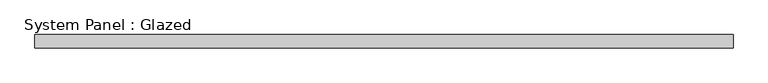
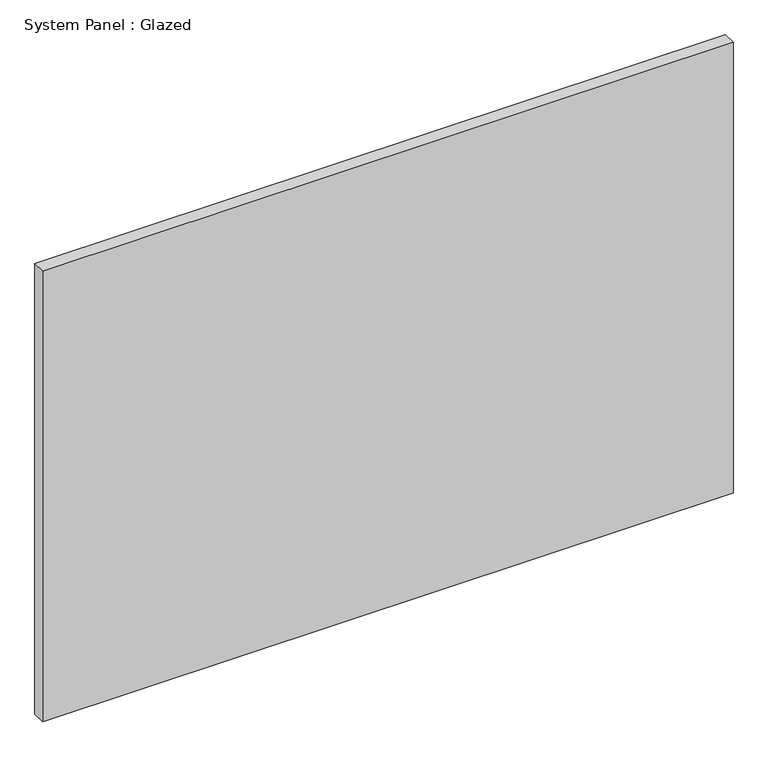
"""IFC4 building model written with IfcOpenShell, lengths in millimetres: plate geometry, System Panel : Glazed."""

from ifc_helpers import new_model, si_unit, origin, origin_with_axes, place, context, project, spatial, polyline, outline, extrude, source, transform, mapped, element, save


def system_panel_glazed_3baabbd8(model_context):
    return source(origin(), model_context, "Body", "SweptSolid", [
        extrude(outline(polyline([(666.7499999, -44.45), (-666.7499999, -44.45), (-666.7499999, -19.05), (666.7499999, -19.05), (666.7499999, -44.45)])), origin_with_axes(), (0.0, 0.0, 1.0), 920.75),
    ])


if __name__ == "__main__":
    model = new_model("IFC4")
    model_context = context("Model", 3, world=origin())
    ifc_project = project(units=[si_unit("LENGTHUNIT", "METRE", prefix="MILLI")], contexts=[model_context])
    site = spatial("IfcSite", under=ifc_project)
    building = spatial("IfcBuilding", under=site)
    placement = place(None, origin())
    system_panel_glazed_shape = system_panel_glazed_3baabbd8(model_context)
    element("IfcPlate", 1, ObjectType="System Panel : Glazed", at=placement, inside=building, context=model_context, shape_type="MappedRepresentation", body=[
        mapped(system_panel_glazed_shape, transform((0.0, 0.0, 0.0), x_axis=(1.0, 0.0, 0.0), y_axis=(0.0, 1.0, 0.0), z_axis=(0.0, 0.0, 1.0))),
    ])
    save(model, "model.ifc")

# Revit data of these elements
# Type "System Panel : Glazed"
#   Construction Type Id = "GSP4R"
#   Analytic Construction = "1/8 in Pilkington single glazing"
#   Visual Light Transmittance = 0.9
#   Solar Heat Gain Coefficient = 0.86
#   Heat Transfer Coefficient (U) = 1.18115 BTU/(h·ft²·°F)
#   Define Thermal Properties by = 1
# Element 1 (IfcPlate, "System Panel : Glazed")
#   Materials on its faces: "glass panel 223"
# Materials
#   "glass panel 223": class "Generic", colour RGB 120 120 120, transparency 0, Cost = 0
